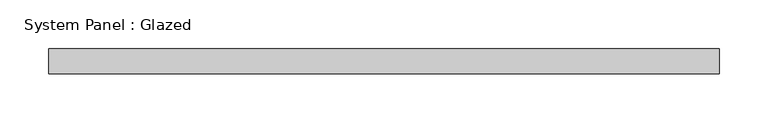
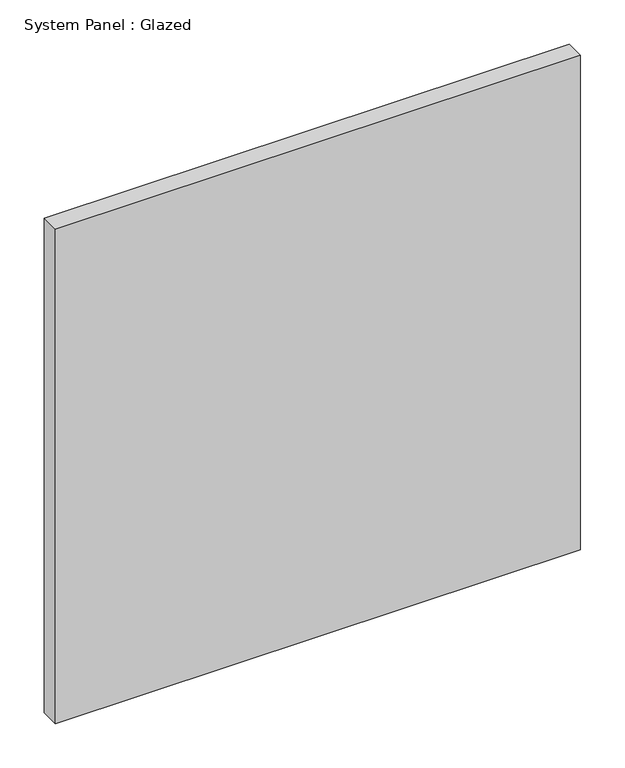
"""IFC4 building model written with IfcOpenShell, lengths in millimetres: plate geometry, System Panel : Glazed."""

from ifc_helpers import new_model, si_unit, origin, origin_with_axes, place, context, project, spatial, polyline, outline, extrude, source, transform, mapped, element, save


def system_panel_glazed_2eb886e8(model_context):
    return source(origin(), model_context, "Body", "SweptSolid", [
        extrude(outline(polyline([(342.9727679, 19.05), (-342.9727679, 19.05), (-342.9727679, 44.45), (342.9727679, 44.45), (342.9727679, 19.05)])), origin_with_axes(), (0.0, 0.0, 1.0), 683.176051),
    ])


if __name__ == "__main__":
    model = new_model("IFC4")
    model_context = context("Model", 3, world=origin())
    ifc_project = project(units=[si_unit("LENGTHUNIT", "METRE", prefix="MILLI")], contexts=[model_context])
    site = spatial("IfcSite", under=ifc_project)
    building = spatial("IfcBuilding", under=site)
    placement = place(None, origin())
    system_panel_glazed_shape = system_panel_glazed_2eb886e8(model_context)
    element("IfcPlate", 1, ObjectType="System Panel : Glazed", at=placement, inside=building, context=model_context, shape_type="MappedRepresentation", body=[
        mapped(system_panel_glazed_shape, transform((0.0, 0.0, 0.0), x_axis=(1.0, 0.0, 0.0), y_axis=(0.0, 1.0, 0.0), z_axis=(0.0, 0.0, 1.0))),
    ])
    save(model, "model.ifc")

# Revit data of these elements
# Type "System Panel : Glazed"
#   Construction Type Id = "GSP4R"
#   Analytic Construction = "1/8 in Pilkington single glazing"
#   Visual Light Transmittance = 0.9
#   Solar Heat Gain Coefficient = 0.86
#   Heat Transfer Coefficient (U) = 1.18115 BTU/(h·ft²·°F)
#   Define Thermal Properties by = 1
# Element 1 (IfcPlate, "System Panel : Glazed")
#   Materials on its faces: "Glass"
# Materials
#   "Glass": class "Glass", colour RGB 0 128 192, transparency 0.75, Description = "Soda Lime Glass", Cost = 0
